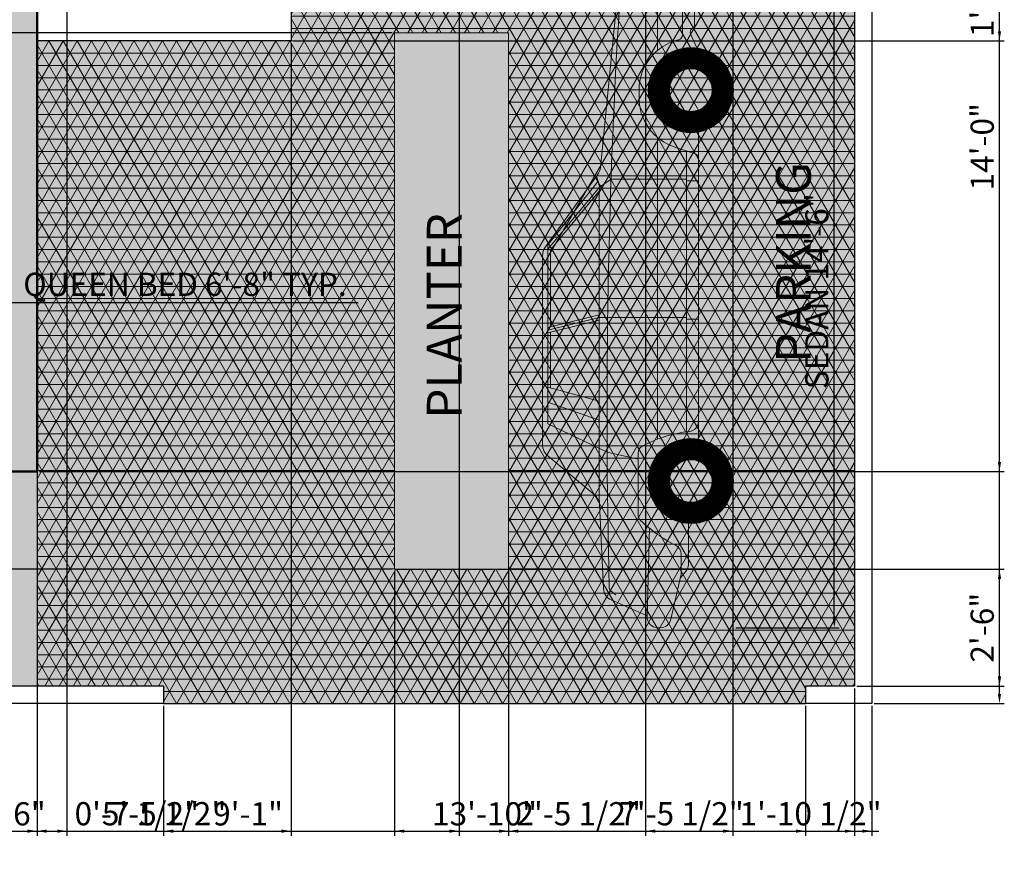
# Model space of a CAD drawing. Units: inches. Extents: x 2623 to 3157, y 1514 to 2273.
# Tile 2 of 6: x 2898 to 3153, y 1514 to 1729. Entities that reach past the tile are written whole.
import ezdxf

# ---------------------------------------------------------------- set-up
doc = ezdxf.new("R2010")
doc.units = ezdxf.units.IN
for name, color, linetype, lineweight in [('A-ANNO-DIMS', 2, 'Continuous', 18), ('A-AREA-IDEN', 7, 'Continuous', 25), ('A-FLOR', 7, 'Continuous', 25), ('A-WALL', 7, 'Continuous', 50), ('A-WALL-PATT', 252, 'Continuous', 13), ('C-PRKG', 8, 'Continuous', 20), ('C-PRKG-BASE-PATT', 51, 'Continuous', 13), ('C-PRKG-PATT', 252, 'Continuous', 13), ('C-PRKG-VEHL', 9, 'Continuous', 13), ('C-PROP', 7, 'Continuous', 25), ('L-PLNT', 3, 'Continuous', 20), ('L-PLNT-PATT', 9, 'Continuous', 13)]:
    doc.layers.add(name, color=color, linetype=linetype, lineweight=lineweight)
doc.styles.get("Standard").update_dxf_attribs({"font": 'arial.ttf'})
doc.dimstyles.new('ISO-25', dxfattribs={"dimtxt": 6, "dimasz": 2.5, "dimexe": 1.25, "dimexo": 0.625, "dimtad": 1, "dimdec": 1, "dimlunit": 3, "dimtxsty": 'Standard', "dimcen": 2.5, "dimadec": 0, "dimazin": 0, "dimtfac": 1, "dimtdec": 1, "dimtmove": 0, "dimatfit": 3, "dimfxl": 1, "dimarcsym": 0})

# ---------------------------------------------------------------- blocks, each defined once
blk = doc.blocks.new('Car - sedan  side')
for p, q in [((-77.81, 49.34), (-126.58, 49.34)), ((-56.87, 35.13), (-75.48, 48.59)), ((-139.53, 35.99), (-129.64, 47.91)), ((-128.57, 32.64), (-121.22, 48.02)), ((-74.7, 48.02), (-121.22, 48.02)), ((-120.32, 34.67), (-115.67, 48.02)), ((-115.4, 34.67), (-111.74, 48.02)), ((-97.55, 47.3), (-111.94, 47.3)), ((-94.41, 34.67), (-97.73, 48.02)), ((-93.72, 34.67), (-97.04, 48.02)), ((-93.03, 34.67), (-96.34, 48.02)), ((-76.26, 47.3), (-96.16, 47.3)), ((-61.08, 34.66), (-76.26, 47.3)), ((-60.02, 34.65), (-76.07, 48.02)), ((-58.54, 34.93), (-74.99, 48.02)), ((-140.23, 34.67), (-163.88, 33.56)), ((-62.28, 34.67), (-140.23, 34.67)), ((-93.72, 19.62), (-93.72, 34.67)), ((-62.28, 34.67), (-60.02, 34.65)), ((-60.02, 34.65), (-58.54, 34.93)), ((-57.97, 31.61), (-60.02, 34.65)), ((-57.21, 35.38), (-58.54, 34.93)), ((-54.93, 34.4), (-8.75, 29.8)), ((-170.93, 22.32), (-166.81, 31.56)), ((-164.57, 31.6), (-165.48, 30.35)), ((-130.39, 24.63), (-128.57, 32.64)), ((-57.97, 19.62), (-57.97, 31.61)), ((-4.21, 24.18), (-5.42, 27.27)), ((-128.78, 24.63), (-144.79, 24.63)), ((-36.97, 24.38), (-34.94, 24.38)), ((-148.26, 21.7), (-171.11, 22.33)), ((-174, 19.51), (-174, 18.91)), ((-47.2, 19.62), (-125.23, 19.62)), ((-93.72, 12.14), (-93.72, 19.62)), ((-57.97, 12.14), (-57.97, 19.62)), ((0, 19.62), (-24.7, 19.62)), ((-160.12, 13.48), (-171.81, 16.16)), ((-159.22, 12.14), (-161.08, 13.7)), ((-155.01, 13.48), (-160.12, 13.48)), ((-51.4, 9.89), (-49.69, 15.14)), ((-4.23, 13.19), (-20.72, 13.19)), ((-9.5, 13.19), (-14.1, 10.2)), ((-3.22, 13.59), (-1.77, 14.97)), ((-147.03, 11.6), (-157.73, 11.6)), ((-50.67, 12.14), (-123.32, 12.14)), ((-94.21, 9.03), (-94.21, 12.14)), ((-58.39, 9.03), (-58.39, 12.14)), ((-20.36, 11.06), (-24.06, 9.44)), ((-18.83, 10.42), (-19.11, 10.76)), ((-120.62, 9.03), (-125.23, 9.03)), ((-45.76, 9.03), (-120.62, 9.03)), ((-14.68, 10.03), (-18.01, 10.03))]:
    blk.add_line(p, q)
at = {"const_width": 5.49}
for points in [[(-127.8, 11, -1), (-144.3, 11, -1)], [(-26.69, 11, -1), (-43.19, 11, -1)]]:
    blk.add_lwpolyline(points, format="xyb", close=True, dxfattribs=at)
for centre, radius in [((-136.05, 11), 11), ((-34.94, 11), 11), ((-136.05, 11), 5.51), ((-34.94, 11), 5.51)]:
    blk.add_circle(centre, radius)
for centre, radius, start, end in [((-126.58, 45.38), 3.97, 90, 140.3029), ((-77.81, 45.38), 3.97, 54.135, 90), ((-142.58, 38.53), 3.97, 272.6827, 320.3029), ((-163.72, 30.18), 3.38, 92.6827, 155.9736), ((-54.54, 38.35), 3.97, 234.135, 264.3123), ((-163.62, 30.91), 1.17, 91.491, 143.9553), ((-118.51, -1702.12), 1734.79, 86.34698, 91.49105), ((-9.15, 25.82), 4, 21.3107, 84.3123), ((-118.09, -2.78), 38.85, 136.3964, 152.9097), ((-144.79, 22.64), 1.98, 90, 136.3964), ((-128.78, 22.64), 1.98, 28.1371, 90), ((-157.14, 7.48), 34.14, 6.5135, 28.1371), ((-36.97, 11), 13.38, 90, 161.9732), ((-34.94, 11), 13.38, 13.5864, 90), ((0.9, 26.18), 5.49, 201.3107, 247.7048), ((-171.18, 19.51), 2.82, 88.4193, 180), ((-1.92, 19.3), 1.94, 325.3744, 67.7048), ((-171.18, 18.91), 2.82, 180, 257.0905), ((2.46, 16.28), 3.37, 145.3744, 172.3839), ((-3.82, 17.12), 2.96, 313.7173, 352.3839), ((-155.01, 16.1), 2.62, 270, 332.9097), ((-20.72, 14.43), 1.24, 193.5864, 270), ((-4.23, 14.65), 1.46, 270, 313.7173), ((-157.73, 13.93), 2.32, 230.1291, 270), ((-120.62, 11.65), 2.62, 186.5135, 270), ((-19.93, 10.09), 1.06, 39.301, 113.7159), ((-18.01, 11.09), 1.06, 219.301, 270), ((-14.68, 11.09), 1.06, 270, 303.047), ((-52.58, 10.27), 1.24, 270, 341.9732)]:
    blk.add_arc(centre, radius, start, end)
blk = doc.blocks.new('*D41')
at = {"layer": 'A-ANNO-DIMS', "color": 0, "lineweight": -2, "transparency": 16777216}
for p, q in [((2813.38, 1667.74), (2813.38, 1655.12)), ((2893.38, 1667.74), (2893.38, 1655.12)), ((2815.88, 1656.37), (2890.88, 1656.37)), ((2893.38, 1656.37), (2985.39, 1656.37))]:
    blk.add_line(p, q, dxfattribs=at)
at = {"layer": 'A-ANNO-DIMS', "color": 0, "transparency": 16777216}
for points in [[(2815.88, 1656.78), (2815.88, 1655.95), (2813.38, 1656.37)], [(2890.88, 1656.78), (2890.88, 1655.95), (2893.38, 1656.37)]]:
    blk.add_solid(points, dxfattribs=at)
at = {"layer": 'Defpoints', "color": 0, "transparency": 16777216}
for p in [(2813.38, 1668.37), (2893.38, 1668.37), (2893.38, 1656.37)]:
    blk.add_point(p, dxfattribs=at)
at = {"layer": 'A-ANNO-DIMS', "color": 0, "transparency": 16777216, "insert": (2940.63, 1660.28), "char_height": 6, "attachment_point": 5}
blk.add_mtext('QUEEN BED 6\'-8" TYP.', dxfattribs=at)
blk = doc.blocks.new('*D57')
at = {"layer": 'A-ANNO-DIMS', "color": 0, "lineweight": -2, "transparency": 16777216}
for p, q in [((3083.08, 1746.36), (3109.82, 1746.36)), ((3108.57, 1574.74), (3108.57, 1743.86)), ((3083.08, 1572.24), (3109.82, 1572.24))]:
    blk.add_line(p, q, dxfattribs=at)
at = {"layer": 'A-ANNO-DIMS', "color": 0, "transparency": 16777216}
for points in [[(3108.16, 1743.86), (3108.99, 1743.86), (3108.57, 1746.36)], [(3108.16, 1574.74), (3108.99, 1574.74), (3108.57, 1572.24)]]:
    blk.add_solid(points, dxfattribs=at)
at = {"layer": 'Defpoints', "color": 0, "transparency": 16777216}
for p in [(3082.46, 1746.36), (3108.57, 1746.36), (3082.46, 1572.24)]:
    blk.add_point(p, dxfattribs=at)
at = {"layer": 'A-ANNO-DIMS', "color": 0, "transparency": 16777216, "insert": (3104.85, 1659.3), "char_height": 6, "attachment_point": 5, "rotation": 90}
blk.add_mtext('SEDAN 14\'-6"', dxfattribs=at)
blk = doc.blocks.new('*D59')
at = {"layer": 'A-ANNO-DIMS', "color": 0, "lineweight": -2, "transparency": 16777216}
for p, q in [((2668.3, 1552.02), (2668.3, 1518.4)), ((3118.3, 1552.02), (3118.3, 1518.4)), ((2670.8, 1519.65), (3115.8, 1519.65))]:
    blk.add_line(p, q, dxfattribs=at)
at = {"layer": 'A-ANNO-DIMS', "color": 0, "transparency": 16777216}
for points in [[(2670.8, 1520.06), (2670.8, 1519.23), (2668.3, 1519.65)], [(3115.8, 1520.06), (3115.8, 1519.23), (3118.3, 1519.65)]]:
    blk.add_solid(points, dxfattribs=at)
at = {"layer": 'Defpoints', "color": 0, "transparency": 16777216}
for p in [(2668.3, 1552.65), (3118.3, 1552.65), (3118.3, 1519.65)]:
    blk.add_point(p, dxfattribs=at)
at = {"layer": 'A-ANNO-DIMS', "color": 0, "transparency": 16777216, "insert": (2893.3, 1523.34), "char_height": 6, "attachment_point": 5}
blk.add_mtext('37\'-6"', dxfattribs=at)
blk = doc.blocks.new('*D60')
at = {"layer": 'A-ANNO-DIMS', "color": 0, "lineweight": -2, "transparency": 16777216}
for p, q in [((3118.92, 2212.65), (3152.55, 2212.65)), ((3151.3, 1555.15), (3151.3, 2210.15)), ((3118.92, 1552.65), (3152.55, 1552.65))]:
    blk.add_line(p, q, dxfattribs=at)
at = {"layer": 'A-ANNO-DIMS', "color": 0, "transparency": 16777216}
for points in [[(3150.88, 2210.15), (3151.71, 2210.15), (3151.3, 2212.65)], [(3150.88, 1555.15), (3151.71, 1555.15), (3151.3, 1552.65)]]:
    blk.add_solid(points, dxfattribs=at)
at = {"layer": 'Defpoints', "color": 0, "transparency": 16777216}
for p in [(3118.3, 2212.65), (3151.3, 2212.65), (3118.3, 1552.65)]:
    blk.add_point(p, dxfattribs=at)
at = {"layer": 'A-ANNO-DIMS', "color": 0, "transparency": 16777216, "insert": (3147.61, 1882.65), "char_height": 6, "attachment_point": 5, "rotation": 90}
blk.add_mtext('55\'-0"', dxfattribs=at)
blk = doc.blocks.new('*D65')
at = {"layer": 'A-ANNO-DIMS', "color": 0, "lineweight": -2, "transparency": 16777216}
for p, q in [((2695.3, 1612.02), (2695.3, 1518.4)), ((2902.38, 1612.02), (2902.38, 1518.4)), ((2697.8, 1519.65), (2899.88, 1519.65))]:
    blk.add_line(p, q, dxfattribs=at)
at = {"layer": 'A-ANNO-DIMS', "color": 0, "transparency": 16777216}
for points in [[(2697.8, 1520.06), (2697.8, 1519.23), (2695.3, 1519.65)], [(2899.88, 1520.06), (2899.88, 1519.23), (2902.38, 1519.65)]]:
    blk.add_solid(points, dxfattribs=at)
at = {"layer": 'Defpoints', "color": 0, "transparency": 16777216}
for p in [(2695.3, 1612.65), (2902.38, 1612.65), (2902.38, 1519.65)]:
    blk.add_point(p, dxfattribs=at)
at = {"layer": 'A-ANNO-DIMS', "color": 0, "transparency": 16777216, "insert": (2798.84, 1523.34), "char_height": 6, "attachment_point": 5}
blk.add_mtext('17\'-3"', dxfattribs=at)
blk = doc.blocks.new('*D66')
at = {"layer": 'A-ANNO-DIMS', "color": 0, "lineweight": -2, "transparency": 16777216}
for p, q in [((2903, 1780.65), (3152.55, 1780.65)), ((3151.3, 1615.15), (3151.3, 1778.15)), ((2903, 1612.65), (3152.55, 1612.65))]:
    blk.add_line(p, q, dxfattribs=at)
at = {"layer": 'A-ANNO-DIMS', "color": 0, "transparency": 16777216}
for points in [[(3150.88, 1778.15), (3151.71, 1778.15), (3151.3, 1780.65)], [(3150.88, 1615.15), (3151.71, 1615.15), (3151.3, 1612.65)]]:
    blk.add_solid(points, dxfattribs=at)
at = {"layer": 'Defpoints', "color": 0, "transparency": 16777216}
for p in [(2902.38, 1780.65), (3151.3, 1780.65), (2902.38, 1612.65)]:
    blk.add_point(p, dxfattribs=at)
at = {"layer": 'A-ANNO-DIMS', "color": 0, "transparency": 16777216, "insert": (3147.61, 1696.65), "char_height": 6, "attachment_point": 5, "rotation": 90}
blk.add_mtext('14\'-0"', dxfattribs=at)
blk = doc.blocks.new('*D67')
at = {"layer": 'A-ANNO-DIMS', "color": 0, "lineweight": -2, "transparency": 16777216}
for p, q in [((2994.86, 1586.75), (2994.86, 1518.4)), ((3024.32, 1586.75), (3024.32, 1518.4)), ((2997.36, 1519.65), (3021.82, 1519.65)), ((3024.32, 1519.65), (3058.1, 1519.65))]:
    blk.add_line(p, q, dxfattribs=at)
at = {"layer": 'A-ANNO-DIMS', "color": 0, "transparency": 16777216}
for points in [[(2997.36, 1520.06), (2997.36, 1519.23), (2994.86, 1519.65)], [(3021.82, 1520.06), (3021.82, 1519.23), (3024.32, 1519.65)]]:
    blk.add_solid(points, dxfattribs=at)
at = {"layer": 'Defpoints', "color": 0, "transparency": 16777216}
for p in [(2994.86, 1587.38), (3024.32, 1587.38), (3024.32, 1519.65)]:
    blk.add_point(p, dxfattribs=at)
at = {"layer": 'A-ANNO-DIMS', "color": 0, "transparency": 16777216, "insert": (3042.46, 1523.37), "char_height": 6, "attachment_point": 5}
blk.add_mtext('2\'-5 1/2"', dxfattribs=at)
blk = doc.blocks.new('*D68')
at = {"layer": 'A-ANNO-DIMS', "color": 0, "lineweight": -2, "transparency": 16777216}
for p, q in [((2994.24, 1726.09), (2634.05, 1726.09)), ((2635.3, 1589.88), (2635.3, 1723.59)), ((2994.24, 1587.38), (2634.05, 1587.38))]:
    blk.add_line(p, q, dxfattribs=at)
at = {"layer": 'A-ANNO-DIMS', "color": 0, "transparency": 16777216}
for points in [[(2634.88, 1723.59), (2635.71, 1723.59), (2635.3, 1726.09)], [(2634.88, 1589.88), (2635.71, 1589.88), (2635.3, 1587.38)]]:
    blk.add_solid(points, dxfattribs=at)
at = {"layer": 'Defpoints', "color": 0, "transparency": 16777216}
for p in [(2635.3, 1726.09), (2994.86, 1726.09), (2994.86, 1587.38)]:
    blk.add_point(p, dxfattribs=at)
at = {"layer": 'A-ANNO-DIMS', "color": 0, "transparency": 16777216, "insert": (2631.57, 1656.73), "char_height": 6, "attachment_point": 5, "rotation": 90}
blk.add_mtext('11\'-6 1/2"', dxfattribs=at)
blk = doc.blocks.new('*D71')
at = {"layer": 'A-ANNO-DIMS', "color": 0, "lineweight": -2, "transparency": 16777216}
for p, q in [((2902.38, 1743.46), (2902.38, 1518.4)), ((3011.52, 1743.46), (3011.52, 1518.4)), ((2904.88, 1519.65), (3009.02, 1519.65))]:
    blk.add_line(p, q, dxfattribs=at)
at = {"layer": 'A-ANNO-DIMS', "color": 0, "transparency": 16777216}
for points in [[(2904.88, 1520.06), (2904.88, 1519.23), (2902.38, 1519.65)], [(3009.02, 1520.06), (3009.02, 1519.23), (3011.52, 1519.65)]]:
    blk.add_solid(points, dxfattribs=at)
at = {"layer": 'Defpoints', "color": 0, "transparency": 16777216}
for p in [(2902.38, 1744.09), (3011.52, 1744.09), (3011.52, 1519.65)]:
    blk.add_point(p, dxfattribs=at)
at = {"layer": 'A-ANNO-DIMS', "color": 0, "transparency": 16777216, "insert": (2956.95, 1523.33), "char_height": 6, "attachment_point": 5}
blk.add_mtext('9\'-1"', dxfattribs=at)
blk = doc.blocks.new('*D73')
at = {"layer": 'A-ANNO-DIMS', "color": 0, "lineweight": -2, "transparency": 16777216}
for p, q in [((2968.72, 1744.09), (3152.55, 1744.09)), ((3151.3, 1726.52), (3151.3, 1741.59)), ((2968.72, 1724.02), (3152.55, 1724.02))]:
    blk.add_line(p, q, dxfattribs=at)
at = {"layer": 'A-ANNO-DIMS', "color": 0, "transparency": 16777216}
for points in [[(3150.88, 1741.59), (3151.71, 1741.59), (3151.3, 1744.09)], [(3150.88, 1726.52), (3151.71, 1726.52), (3151.3, 1724.02)]]:
    blk.add_solid(points, dxfattribs=at)
at = {"layer": 'Defpoints', "color": 0, "transparency": 16777216}
for p in [(2968.09, 1744.09), (3151.3, 1744.09), (2968.09, 1724.02)]:
    blk.add_point(p, dxfattribs=at)
at = {"layer": 'A-ANNO-DIMS', "color": 0, "transparency": 16777216, "insert": (3147.61, 1734.05), "char_height": 6, "attachment_point": 5, "rotation": 90}
blk.add_mtext('1\'-8"', dxfattribs=at)
blk = doc.blocks.new('*D74')
at = {"layer": 'A-ANNO-DIMS', "color": 0, "lineweight": -2, "transparency": 16777216}
for p, q in [((2902.38, 1723.39), (2902.38, 1518.4)), ((2968.09, 1723.39), (2968.09, 1518.4)), ((2904.88, 1519.65), (2965.59, 1519.65))]:
    blk.add_line(p, q, dxfattribs=at)
at = {"layer": 'A-ANNO-DIMS', "color": 0, "transparency": 16777216}
for points in [[(2904.88, 1520.06), (2904.88, 1519.23), (2902.38, 1519.65)], [(2965.59, 1520.06), (2965.59, 1519.23), (2968.09, 1519.65)]]:
    blk.add_solid(points, dxfattribs=at)
at = {"layer": 'Defpoints', "color": 0, "transparency": 16777216}
for p in [(2902.38, 1724.02), (2968.09, 1724.02), (2968.09, 1519.65)]:
    blk.add_point(p, dxfattribs=at)
at = {"layer": 'A-ANNO-DIMS', "color": 0, "transparency": 16777216, "insert": (2935.23, 1523.37), "char_height": 6, "attachment_point": 5}
blk.add_mtext('5\'-5 1/2"', dxfattribs=at)
blk = doc.blocks.new('*D75')
at = {"layer": 'A-ANNO-DIMS', "color": 0, "lineweight": -2, "transparency": 16777216}
for p, q in [((3024.32, 1586.75), (3024.32, 1518.4)), ((3113.8, 1556.52), (3113.8, 1518.4)), ((3026.82, 1519.65), (3111.3, 1519.65))]:
    blk.add_line(p, q, dxfattribs=at)
at = {"layer": 'A-ANNO-DIMS', "color": 0, "transparency": 16777216}
for points in [[(3026.82, 1520.06), (3026.82, 1519.23), (3024.32, 1519.65)], [(3111.3, 1520.06), (3111.3, 1519.23), (3113.8, 1519.65)]]:
    blk.add_solid(points, dxfattribs=at)
at = {"layer": 'Defpoints', "color": 0, "transparency": 16777216}
for p in [(3024.32, 1587.38), (3113.8, 1557.15), (3113.8, 1519.65)]:
    blk.add_point(p, dxfattribs=at)
at = {"layer": 'A-ANNO-DIMS', "color": 0, "transparency": 16777216, "insert": (3069.06, 1523.37), "char_height": 6, "attachment_point": 5}
blk.add_mtext('7\'-5 1/2"', dxfattribs=at)
blk = doc.blocks.new('*D81')
at = {"layer": 'A-ANNO-DIMS', "color": 0, "lineweight": -2, "transparency": 16777216}
for p, q in [((2935.08, 1552.02), (2935.08, 1518.4)), ((3101.15, 1552.02), (3101.15, 1518.4)), ((2937.58, 1519.65), (3098.65, 1519.65))]:
    blk.add_line(p, q, dxfattribs=at)
at = {"layer": 'A-ANNO-DIMS', "color": 0, "transparency": 16777216}
for points in [[(2937.58, 1520.06), (2937.58, 1519.23), (2935.08, 1519.65)], [(3098.65, 1520.06), (3098.65, 1519.23), (3101.15, 1519.65)]]:
    blk.add_solid(points, dxfattribs=at)
at = {"layer": 'Defpoints', "color": 0, "transparency": 16777216}
for p in [(2935.08, 1552.65), (3101.15, 1552.65), (3101.15, 1519.65)]:
    blk.add_point(p, dxfattribs=at)
at = {"layer": 'A-ANNO-DIMS', "color": 0, "transparency": 16777216, "insert": (3018.11, 1523.34), "char_height": 6, "attachment_point": 5}
blk.add_mtext('13\'-10"', dxfattribs=at)
blk = doc.blocks.new('*D82')
at = {"layer": 'A-ANNO-DIMS', "color": 0, "lineweight": -2, "transparency": 16777216}
for p, q in [((2995.49, 1587.38), (3152.55, 1587.38)), ((3151.3, 1559.65), (3151.3, 1584.88)), ((3114.42, 1557.15), (3152.55, 1557.15))]:
    blk.add_line(p, q, dxfattribs=at)
at = {"layer": 'A-ANNO-DIMS', "color": 0, "transparency": 16777216}
for points in [[(3150.88, 1584.88), (3151.71, 1584.88), (3151.3, 1587.38)], [(3150.88, 1559.65), (3151.71, 1559.65), (3151.3, 1557.15)]]:
    blk.add_solid(points, dxfattribs=at)
at = {"layer": 'Defpoints', "color": 0, "transparency": 16777216}
for p in [(2994.86, 1587.38), (3151.3, 1587.38), (3113.8, 1557.15)]:
    blk.add_point(p, dxfattribs=at)
at = {"layer": 'A-ANNO-DIMS', "color": 0, "transparency": 16777216, "insert": (3147.61, 1572.26), "char_height": 6, "attachment_point": 5, "rotation": 90}
blk.add_mtext('2\'-6"', dxfattribs=at)
blk = doc.blocks.new('*D83')
at = {"layer": 'A-ANNO-DIMS', "color": 0, "lineweight": -2, "transparency": 16777216}
for p, q in [((2902.38, 1780.02), (2902.38, 1518.4)), ((2910.08, 1780.02), (2910.08, 1518.4)), ((2904.88, 1519.65), (2907.58, 1519.65)), ((2910.08, 1519.65), (2943.76, 1519.65))]:
    blk.add_line(p, q, dxfattribs=at)
at = {"layer": 'A-ANNO-DIMS', "color": 0, "transparency": 16777216}
for points in [[(2904.88, 1520.06), (2904.88, 1519.23), (2902.38, 1519.65)], [(2907.58, 1520.06), (2907.58, 1519.23), (2910.08, 1519.65)]]:
    blk.add_solid(points, dxfattribs=at)
at = {"layer": 'Defpoints', "color": 0, "transparency": 16777216}
for p in [(2902.38, 1780.65), (2910.08, 1780.65), (2910.08, 1519.65)]:
    blk.add_point(p, dxfattribs=at)
at = {"layer": 'A-ANNO-DIMS', "color": 0, "transparency": 16777216, "insert": (2928.17, 1523.37), "char_height": 6, "attachment_point": 5}
blk.add_mtext('0\'-7 1/2"', dxfattribs=at)
blk = doc.blocks.new('*D84')
at = {"layer": 'A-ANNO-DIMS', "color": 0, "lineweight": -2, "transparency": 16777216}
for p, q in [((3059.78, 1780.02), (3059.78, 1518.4)), ((3082.3, 1780.02), (3082.3, 1518.4)), ((3062.28, 1519.65), (3079.8, 1519.65)), ((3082.3, 1519.65), (3120.07, 1519.65))]:
    blk.add_line(p, q, dxfattribs=at)
at = {"layer": 'A-ANNO-DIMS', "color": 0, "transparency": 16777216}
for points in [[(3062.28, 1520.06), (3062.28, 1519.23), (3059.78, 1519.65)], [(3079.8, 1520.06), (3079.8, 1519.23), (3082.3, 1519.65)]]:
    blk.add_solid(points, dxfattribs=at)
at = {"layer": 'Defpoints', "color": 0, "transparency": 16777216}
for p in [(3059.78, 1780.65), (3082.3, 1780.65), (3082.3, 1519.65)]:
    blk.add_point(p, dxfattribs=at)
at = {"layer": 'A-ANNO-DIMS', "color": 0, "transparency": 16777216, "insert": (3102.43, 1523.37), "char_height": 6, "attachment_point": 5}
blk.add_mtext('1\'-10 1/2"', dxfattribs=at)

msp = doc.modelspace()

# ---------------------------------------------------------------- hatches: boundary and pattern name
at = {"layer": 'A-WALL-PATT'}
h = msp.add_hatch(color=256, dxfattribs=at)
h.dxf.hatch_style = 1
h.paths.add_polyline_path([(3082.3, 1813.09), (3073.3, 1813.09), (3073.3, 1789.65), (3059.78, 1789.65), (3059.78, 1780.65), (3082.3, 1780.65)])
h.paths.add_polyline_path([(2969.78, 1789.65), (2946.08, 1789.65), (2946.08, 1780.65), (2969.78, 1780.65)])
h.paths.add_polyline_path([(2910.08, 1789.65), (2902.38, 1789.65), (2902.38, 1814.02), (2893.38, 1814.02), (2893.38, 1621.65), (2854.7, 1621.65), (2854.7, 1612.65), (2902.38, 1612.65), (2902.38, 1780.65), (2910.08, 1780.65)])
at = {"layer": 'C-PRKG-BASE-PATT'}
h = msp.add_hatch(color=256, dxfattribs=at)
h.dxf.hatch_style = 1
h.paths.add_polyline_path([(3113.8, 1780.65), (3082.3, 1780.65), (3011.52, 1780.65), (3011.52, 1744.09), (2968.09, 1744.09), (2968.09, 1724.02), (2902.38, 1724.02), (2902.38, 1557.15), (2935.08, 1557.15), (2935.08, 1552.65), (3101.15, 1552.65), (3101.15, 1557.15), (3113.8, 1557.15)])
h.paths.add_polyline_path([(3024.32, 1587.38), (2994.86, 1587.38), (2994.86, 1726.09), (3024.32, 1726.09)], flags=16)
h.paths.add_polyline_path([(3017.09, 1623.1), (3017.09, 1685.59), (2998.55, 1685.59), (2998.55, 1623.1)], flags=8)
at = {"layer": 'C-PRKG-PATT'}
h = msp.add_hatch(dxfattribs=at)
h.set_pattern_fill('NET3', color=256)
h.paths.add_polyline_path([(3113.8, 1780.65), (3082.3, 1780.65), (3011.52, 1780.65), (3011.52, 1744.09), (2968.09, 1744.09), (2968.09, 1724.02), (2902.38, 1724.02), (2902.38, 1557.15), (2935.08, 1557.15), (2935.08, 1552.65), (3101.15, 1552.65), (3101.15, 1557.15), (3113.8, 1557.15)])
h.paths.add_polyline_path([(2994.86, 1726.09), (3024.32, 1726.09), (3024.32, 1587.38), (2994.86, 1587.38)], flags=16)
h.paths.add_polyline_path([(3017.09, 1623.1), (3017.09, 1685.59), (2998.55, 1685.59), (2998.55, 1623.1)], flags=8)
at = {"layer": 'L-PLNT-PATT'}
h = msp.add_hatch(color=256, dxfattribs=at)
h.dxf.hatch_style = 1
h.set_gradient(color1=(19, 155, 72), color2=(63, 255, 0), name='CURVED')
h.paths.add_polyline_path([(2902.38, 1612.65), (2695.3, 1612.65), (2695.3, 2185.65), (3082.3, 2185.65), (3082.3, 1780.65), (3113.8, 1780.65), (3113.8, 2208.15), (2672.8, 2208.15), (2672.8, 1557.15), (2902.38, 1557.15)])
h = msp.add_hatch(color=256, dxfattribs=at)
h.dxf.hatch_style = 1
h.set_gradient(color1=(19, 155, 72), color2=(63, 255, 0), name='CYLINDER')
h.paths.add_polyline_path([(3024.32, 1726.09), (2994.86, 1726.09), (2994.86, 1587.38), (3024.32, 1587.38)], flags=17)
h.paths.add_polyline_path([(2902.38, 1612.65), (2695.3, 1612.65), (2695.3, 2185.65), (3082.3, 2185.65), (3082.3, 1780.65), (3113.8, 1780.65), (3113.8, 2208.15), (2672.8, 2208.15), (2672.8, 1557.15), (2902.38, 1557.15)])
h = msp.add_hatch(color=256, dxfattribs=at)
h.dxf.hatch_style = 1
h.set_gradient(color1=(19, 155, 72), color2=(63, 255, 0), name='CURVED')
h.paths.add_polyline_path([(3024.32, 1726.09), (2994.86, 1726.09), (2994.86, 1587.38), (3024.32, 1587.38)])
h.paths.add_polyline_path([(3020.4, 1621.55), (3020.4, 1684.04), (3001.85, 1684.04), (3001.85, 1621.55)], flags=24)

# ---------------------------------------------------------------- linework, layer by layer
at = {"layer": 'A-FLOR'}
for p, q in [((2968.09, 1744.09), (2968.09, 1724.02)), ((2968.09, 1724.02), (2902.38, 1724.02))]:
    msp.add_line(p, q, dxfattribs=at)
msp.add_lwpolyline([(2902.38, 1744.09), (2968.09, 1744.09), (2968.09, 1724.02), (2902.38, 1724.02)], close=True, dxfattribs=at)
at = {"layer": 'A-WALL'}
for q in [(2902.38, 1780.65), (2695.3, 1612.65)]:
    msp.add_line((2902.38, 1612.65), q, dxfattribs=at)
at = {"layer": 'C-PRKG'}
for p, q in [((3113.8, 1557.15), (3113.8, 1780.65)), ((2902.38, 1724.02), (2902.38, 1557.15)), ((2902.38, 1557.15), (2935.08, 1557.15)), ((3101.15, 1557.15), (3113.8, 1557.15))]:
    msp.add_line(p, q, dxfattribs=at)
at = {"layer": 'C-PROP'}
for p, q in [((3118.3, 2212.65), (3118.3, 1552.65)), ((3113.8, 2208.15), (3113.8, 1557.15)), ((2935.08, 1557.15), (2672.8, 1557.15)), ((2935.08, 1557.15), (2935.08, 1552.65)), ((3113.8, 1557.15), (3101.15, 1557.15)), ((3101.15, 1557.15), (3101.15, 1552.65)), ((2935.08, 1552.65), (2668.3, 1552.65)), ((2935.08, 1552.65), (3101.15, 1552.65)), ((3118.3, 1552.65), (3101.15, 1552.65))]:
    msp.add_line(p, q, dxfattribs=at)
at = {"layer": 'L-PLNT'}
for p, q in [((2994.86, 1587.38), (2994.86, 1726.09)), ((2994.86, 1726.09), (3024.32, 1726.09)), ((3024.32, 1726.09), (3024.32, 1587.38))]:
    msp.add_line(p, q, dxfattribs=at)
msp.add_lwpolyline([(2994.86, 1726.09), (3024.32, 1726.09), (3024.32, 1587.38), (2994.86, 1587.38)], close=True, dxfattribs=at)

# ---------------------------------------------------------------- block references
at = {"layer": 'C-PRKG-VEHL', "rotation": 90}
msp.add_blockref('Car - sedan  side', (3082.46, 1746.24), dxfattribs=at)

# ---------------------------------------------------------------- texts
at = {"layer": 'A-AREA-IDEN', "char_height": 9, "width": 50.0068, "attachment_point": 1, "rotation": 90}
for s, insert in [('PARKING', (3093.5, 1640.76)), ('PLANTER', (3003.18, 1626.32))]:
    msp.add_mtext(s, dxfattribs=dict(at, insert=insert))

# ---------------------------------------------------------------- dimensions: what is measured, and where the dimension line sits
at = {"layer": 'A-ANNO-DIMS'}
for base, p1, p2, picture, middle in [((3151.3, 2212.65), (3118.3, 1552.65), (3118.3, 2212.65), '*D60', (3147.61, 1882.65)), ((3151.3, 1780.65), (2902.38, 1612.65), (2902.38, 1780.65), '*D66', (3147.61, 1696.65)), ((3151.3, 1744.09), (2968.09, 1724.02), (2968.09, 1744.09), '*D73', (3147.61, 1734.05)), ((2635.3, 1726.09), (2994.86, 1587.38), (2994.86, 1726.09), '*D68', (2631.57, 1656.73)), ((3151.3, 1587.38), (3113.8, 1557.15), (2994.86, 1587.38), '*D82', (3147.61, 1572.26))]:
    dim = msp.add_linear_dim(base=base, p1=p1, p2=p2, angle=90, dimstyle='ISO-25', override={"dimdec": 1, "dimlfac": 1, "dimrnd": 0, "dimzin": 1, "dimdsep": 46, "dimlunit": 4, "dimfrac": 2}, dxfattribs=at)
    dim.commit()
    dim.dimension.update_dxf_attribs({"geometry": picture, "text_midpoint": middle})
for base, p1, p2, picture, middle in [((2910.08, 1519.65), (2902.38, 1780.65), (2910.08, 1780.65), '*D83', (2928.17, 1523.37)), ((3082.3, 1519.65), (3059.78, 1780.65), (3082.3, 1780.65), '*D84', (3102.43, 1523.37)), ((3011.52, 1519.65), (2902.38, 1744.09), (3011.52, 1744.09), '*D71', (2956.95, 1523.33)), ((2968.09, 1519.65), (2902.38, 1724.02), (2968.09, 1724.02), '*D74', (2935.23, 1523.37)), ((2902.38, 1519.65), (2695.3, 1612.65), (2902.38, 1612.65), '*D65', (2798.84, 1523.34)), ((3024.32, 1519.65), (2994.86, 1587.38), (3024.32, 1587.38), '*D67', (3042.46, 1523.37)), ((3113.8, 1519.65), (3024.32, 1587.38), (3113.8, 1557.15), '*D75', (3069.06, 1523.37)), ((3118.3, 1519.65), (2668.3, 1552.65), (3118.3, 1552.65), '*D59', (2893.3, 1523.34)), ((3101.15, 1519.65), (2935.08, 1552.65), (3101.15, 1552.65), '*D81', (3018.11, 1523.34))]:
    dim = msp.add_linear_dim(base=base, p1=p1, p2=p2, dimstyle='ISO-25', override={"dimdec": 1, "dimlfac": 1, "dimrnd": 0, "dimzin": 1, "dimdsep": 46, "dimlunit": 4, "dimfrac": 2}, dxfattribs=at)
    dim.commit()
    dim.dimension.update_dxf_attribs({"geometry": picture, "text_midpoint": middle})
dim = msp.add_linear_dim(base=(3108.57, 1746.36), p1=(3082.46, 1572.24), p2=(3082.46, 1746.36), angle=90, text='SEDAN <>', dimstyle='ISO-25', override={"dimdec": 1, "dimlfac": 1, "dimrnd": 0, "dimzin": 1, "dimdsep": 46, "dimlunit": 4, "dimfrac": 2}, dxfattribs=at)
dim.commit()
dim.dimension.update_dxf_attribs({"geometry": '*D57', "text_midpoint": (3104.85, 1659.3)})
dim = msp.add_linear_dim(base=(2893.38, 1656.37), p1=(2813.38, 1668.37), p2=(2893.38, 1668.37), text='QUEEN BED <> TYP.', dimstyle='ISO-25', override={"dimdec": 1, "dimlfac": 1, "dimrnd": 0, "dimzin": 1, "dimdsep": 46, "dimlunit": 4, "dimfrac": 2}, dxfattribs=at)
dim.commit()
dim.dimension.update_dxf_attribs({"geometry": '*D41', "text_midpoint": (2940.63, 1660.28)})

doc.saveas('drawing.dxf')
